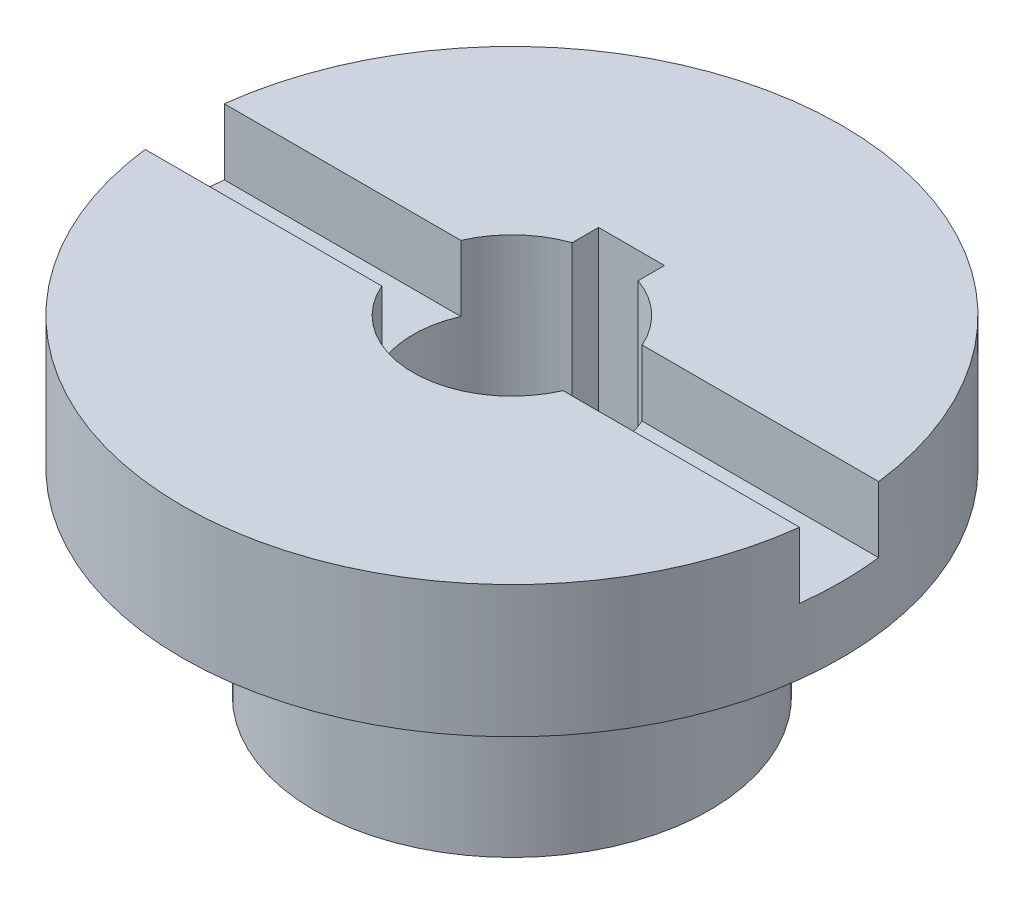
SolidWorks part; units mm, degrees
material "Plain Carbon Steel"
ref_plane "Front Plane" through (0, 0, 0) normal (0, 0, 1) x (1, 0, 0)
ref_plane "Top Plane" through (0, 0, 0) normal (0, 1, 0) x (1, 0, 0)
ref_plane "Right Plane" through (0, 0, 0) normal (1, 0, 0) x (0, 0, -1)
sketch "Flange Profile Sketch" plane through (0, 0, 0) normal (0, 0, 1) x (1, 0, 0)
  line L0 (0, 54.1188) -> (0, -68.6782) construction
  line L1 (0, 0) -> (50, 0)
  line L2 (50, 0) -> (50, -20)
  line L3 (50, -20) -> (33, -20)
  line L4 (30, -23) -> (30, -50)
  line L5 (30, -50) -> (0, -50)
  line L6 (0, -50) -> (0, 0)
  arc A0 (30, -23) -> (33, -20) centre (33, -23) cw
  point P12 (30, -20)
  dimension "D5" = 3
  dimension "D1" = 50
  dimension "D2" = 30
  dimension "D3" = 20
  dimension "D4" = 30
revolve "Flange Body Revolve" add sketch "Flange Profile Sketch" angle 360 about L0
sketch "Bore Keyway Sketch" plane through (0, 0, 0) normal (0, 1, 0) x (1, 0, 0)
  line L0 (0, 54.1221) -> (0, -54.0206) construction
  line L3 (-5, 14.1421) -> (-5, 18.1421)
  line L4 (-5, 18.1421) -> (5, 18.1421)
  line L5 (5, 14.1421) -> (5, 18.1421)
  arc A0 (-5, 14.1421) -> (5, 14.1421) centre (0, 0) ccw
  point P5 (0, 15)
  dimension "D1" = 30
  dimension "D2" = 4
  dimension "D3" = 10
  dimension "D4" = 18.1421
extrude "Bore Keyway 4mm" cut sketch "Bore Keyway Sketch" against normal through all
sketch "Cross Slot Sketch" plane through (0, 0, 0) normal (0, 1, 0) x (1, 0, 0)
  line L0 (-61.3573, 0) -> (63.8616, 0) construction
  line L2 (-59.6877, -6) -> (59.6877, -6)
  line L3 (-59.6877, -6) -> (-59.6877, 6)
  line L4 (-59.6877, 6) -> (59.6877, 6)
  line L5 (59.6877, -6) -> (59.6877, 6)
  line L6 (-59.6877, -6) -> (59.6877, 6) construction
  line L7 (-59.6877, 6) -> (59.6877, -6) construction
  point P3 (0, 0)
  dimension "D1" = 12
  dimension "D2" = 119.3753
extrude "Cross Slot 12x10" cut sketch "Cross Slot Sketch" against normal blind 10
